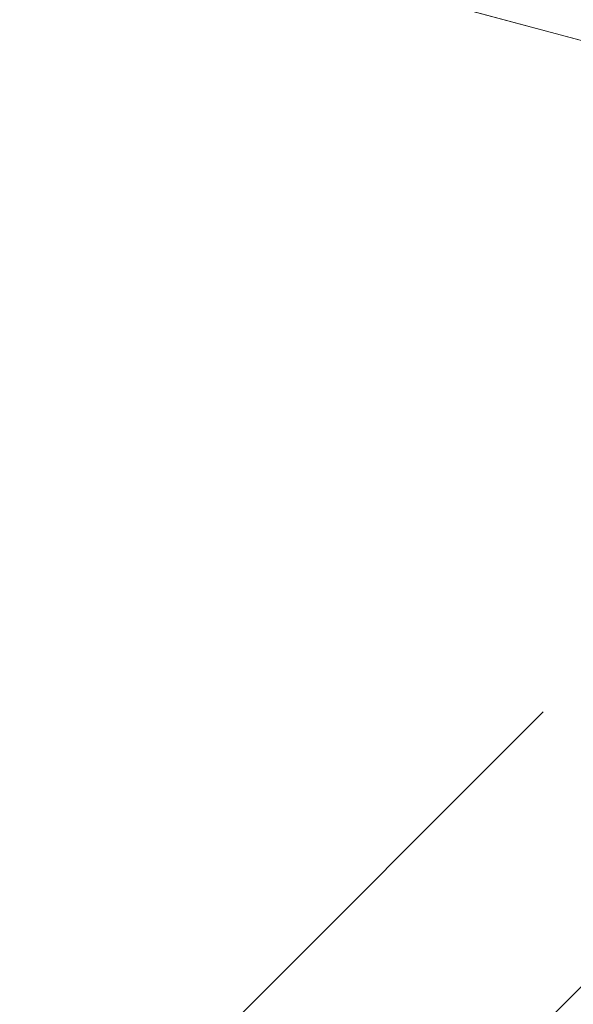
# Model space of a CAD drawing. Units: inches. Extents: x 375 to 1122, y 27 to 1069.
# Tile 51 of 155: x 723.474 to 725.537, y 308.183 to 311.85. Entities that reach past the tile are written whole.
import ezdxf

# ---------------------------------------------------------------- set-up
doc = ezdxf.new("R2010")
doc.units = ezdxf.units.IN
doc.layers.add('Furniture', color=30, linetype='Continuous', lineweight=18)

# ---------------------------------------------------------------- blocks, each defined once
blk = doc.blocks.new('A$C403C54AD')
for p, q in [((0.906853, 1.059765, -0.000599), (1.019435, 0.947232, -0.000599)), ((0.925555, 1.011934, -0.000599), (1.038137, 0.8994, -0.000599))]:
    blk.add_line(p, q)
at = {"linetype": 'ByBlock', "invisible_edges": 5}
for points in [[(0.818605, 0.976049, -0.033549), (0.847931, 0.959118, -0.024314), (0.86649, 1.028382, -0.024314), (0.832628, 1.028382, -0.033549)], [(0.847931, 0.959118, -0.019696), (0.831935, 0.968354, -0.019696), (0.84802, 1.028382, -0.019696), (0.86649, 1.028382, -0.019696)]]:
    blk.add_3dface(points, dxfattribs=at)
at = {"linetype": 'ByBlock'}
blk.add_3dface([(0.847931, 0.959118, -0.024314), (0.847931, 0.959118, -0.019696), (0.86649, 1.028382, -0.019696), (0.86649, 1.028382, -0.024314)], dxfattribs=at)

msp = doc.modelspace()

# ---------------------------------------------------------------- block references
at = {"layer": 'Furniture', "xscale": 39.9918517141215, "yscale": 39.9918517141215, "zscale": 39.9918517141215, "rotation": 270}
msp.add_blockref('A$C403C54AD', (684.9549, 346.2875, 0.024), dxfattribs=at)

doc.saveas('drawing.dxf')
